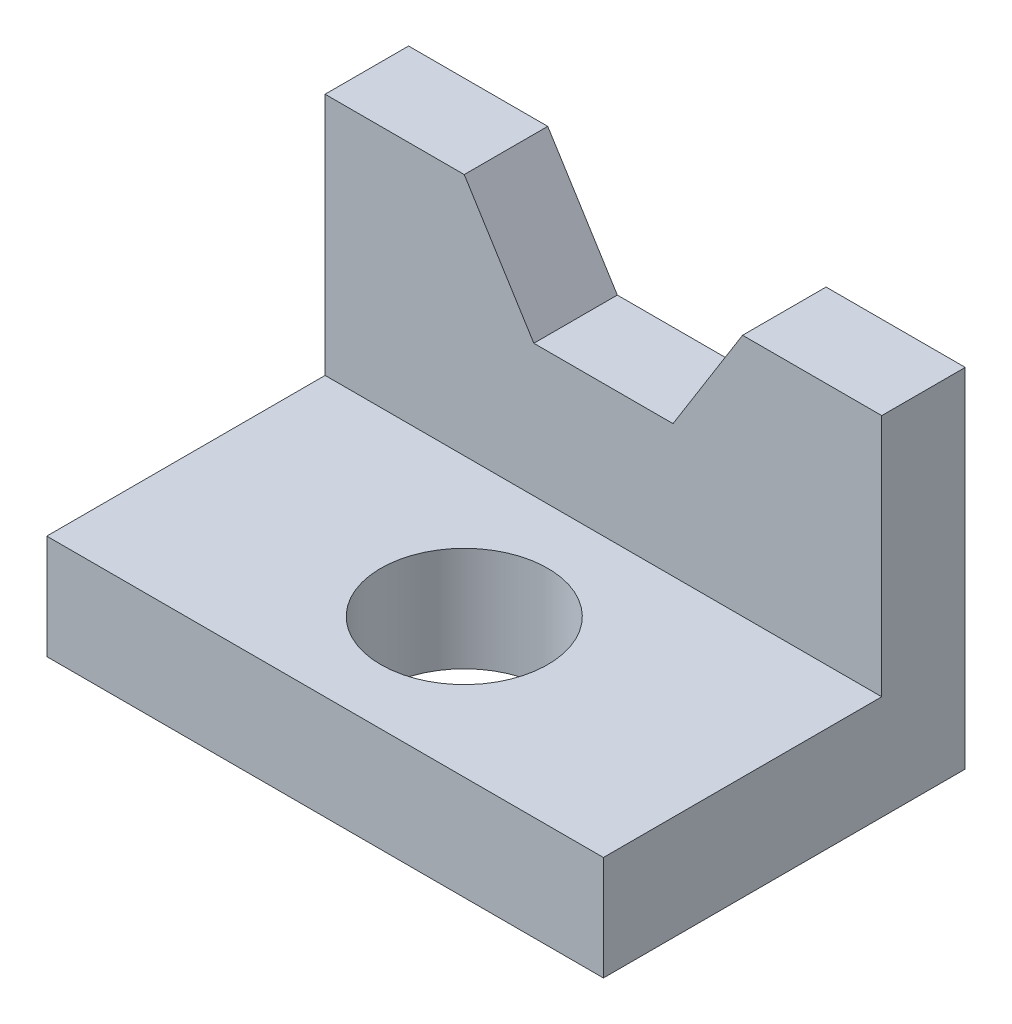
ISO-10303-21;
HEADER;
FILE_DESCRIPTION(('STEP AP214'),'2;1');
FILE_NAME('part.step','',(''),(''),'','','');
FILE_SCHEMA(('AUTOMOTIVE_DESIGN { 1 0 10303 214 1 1 1 1 }'));
ENDSEC;
DATA;
#1=APPLICATION_CONTEXT('core data for automotive mechanical design processes');
#2=APPLICATION_PROTOCOL_DEFINITION('international standard','automotive_design',2000,#1);
#3=PRODUCT_CONTEXT('',#1,'mechanical');
#4=PRODUCT('Part','Part','',(#3));
#5=PRODUCT_RELATED_PRODUCT_CATEGORY('part','',(#4));
#6=PRODUCT_DEFINITION_FORMATION('','',#4);
#7=PRODUCT_DEFINITION_CONTEXT('part definition',#1,'design');
#8=PRODUCT_DEFINITION('design','',#6,#7);
#9=PRODUCT_DEFINITION_SHAPE('','',#8);
#10=(LENGTH_UNIT() NAMED_UNIT(*) SI_UNIT(.MILLI.,.METRE.));
#11=(NAMED_UNIT(*) PLANE_ANGLE_UNIT() SI_UNIT($,.RADIAN.));
#12=(NAMED_UNIT(*) SI_UNIT($,.STERADIAN.) SOLID_ANGLE_UNIT());
#13=UNCERTAINTY_MEASURE_WITH_UNIT(LENGTH_MEASURE(1.E-05),#10,'distance_accuracy_value','');
#14=(GEOMETRIC_REPRESENTATION_CONTEXT(3) GLOBAL_UNCERTAINTY_ASSIGNED_CONTEXT((#13)) GLOBAL_UNIT_ASSIGNED_CONTEXT((#10,
#11,#12)) REPRESENTATION_CONTEXT('',''));
#15=CARTESIAN_POINT('',(0.,0.,0.));
#16=DIRECTION('',(0.,0.,1.));
#17=DIRECTION('',(1.,0.,0.));
#18=AXIS2_PLACEMENT_3D('',#15,#16,#17);
#19=CARTESIAN_POINT('',(0.,0.,12.));
#20=DIRECTION('',(0.,-1.,0.));
#21=DIRECTION('',(0.,0.,-1.));
#22=AXIS2_PLACEMENT_3D('',#19,#20,#21);
#23=PLANE('',#22);
#24=DIRECTION('',(-1.,0.,0.));
#25=VECTOR('',#24,1.);
#26=CARTESIAN_POINT('',(0.,0.,0.));
#27=LINE('',#26,#25);
#28=CARTESIAN_POINT('',(20.,0.,0.));
#29=VERTEX_POINT('',#28);
#30=CARTESIAN_POINT('',(0.,0.,0.));
#31=VERTEX_POINT('',#30);
#32=EDGE_CURVE('E143',#29,#31,#27,.T.);
#33=ORIENTED_EDGE('',*,*,#32,.T.);
#34=DIRECTION('',(0.,0.,-1.));
#35=VECTOR('',#34,1.);
#36=CARTESIAN_POINT('',(0.,0.,12.));
#37=LINE('',#36,#35);
#38=CARTESIAN_POINT('',(0.,0.,12.));
#39=VERTEX_POINT('',#38);
#40=EDGE_CURVE('E11',#39,#31,#37,.T.);
#41=ORIENTED_EDGE('',*,*,#40,.F.);
#42=DIRECTION('',(-1.,0.,0.));
#43=VECTOR('',#42,1.);
#44=CARTESIAN_POINT('',(0.,0.,12.));
#45=LINE('',#44,#43);
#46=CARTESIAN_POINT('',(20.,0.,12.));
#47=VERTEX_POINT('',#46);
#48=EDGE_CURVE('E160',#47,#39,#45,.T.);
#49=ORIENTED_EDGE('',*,*,#48,.F.);
#50=DIRECTION('',(0.,0.,-1.));
#51=VECTOR('',#50,1.);
#52=CARTESIAN_POINT('',(20.,0.,12.));
#53=LINE('',#52,#51);
#54=EDGE_CURVE('E140',#47,#29,#53,.T.);
#55=ORIENTED_EDGE('',*,*,#54,.T.);
#56=EDGE_LOOP('',(#33,#41,#49,#55));
#57=FACE_BOUND('',#56,.T.);
#58=ADVANCED_FACE('F41',(#57),#23,.F.);
#59=CARTESIAN_POINT('',(0.,0.,12.));
#60=DIRECTION('',(1.,0.,0.));
#61=DIRECTION('',(0.,0.,-1.));
#62=AXIS2_PLACEMENT_3D('',#59,#60,#61);
#63=PLANE('',#62);
#64=DIRECTION('',(0.,-1.,0.));
#65=VECTOR('',#64,1.);
#66=CARTESIAN_POINT('',(0.,0.,0.));
#67=LINE('',#66,#65);
#68=CARTESIAN_POINT('',(0.,-50.,0.));
#69=VERTEX_POINT('',#68);
#70=EDGE_CURVE('E145',#31,#69,#67,.T.);
#71=ORIENTED_EDGE('',*,*,#70,.T.);
#72=DIRECTION('',(0.,0.,-1.));
#73=VECTOR('',#72,1.);
#74=CARTESIAN_POINT('',(0.,-50.,12.));
#75=LINE('',#74,#73);
#76=CARTESIAN_POINT('',(0.,-50.,52.));
#77=VERTEX_POINT('',#76);
#78=EDGE_CURVE('E48',#77,#69,#75,.T.);
#79=ORIENTED_EDGE('',*,*,#78,.F.);
#80=DIRECTION('',(0.,-1.,0.));
#81=VECTOR('',#80,1.);
#82=CARTESIAN_POINT('',(0.,-50.,52.));
#83=LINE('',#82,#81);
#84=CARTESIAN_POINT('',(0.,-35.,52.));
#85=VERTEX_POINT('',#84);
#86=EDGE_CURVE('E199',#85,#77,#83,.T.);
#87=ORIENTED_EDGE('',*,*,#86,.F.);
#88=DIRECTION('',(0.,0.,-1.));
#89=VECTOR('',#88,1.);
#90=CARTESIAN_POINT('',(0.,-35.,52.));
#91=LINE('',#90,#89);
#92=CARTESIAN_POINT('',(0.,-35.,12.));
#93=VERTEX_POINT('',#92);
#94=EDGE_CURVE('E198',#85,#93,#91,.T.);
#95=ORIENTED_EDGE('',*,*,#94,.T.);
#96=DIRECTION('',(0.,-1.,0.));
#97=VECTOR('',#96,1.);
#98=CARTESIAN_POINT('',(0.,0.,12.));
#99=LINE('',#98,#97);
#100=EDGE_CURVE('E103',#39,#93,#99,.T.);
#101=ORIENTED_EDGE('',*,*,#100,.F.);
#102=ORIENTED_EDGE('',*,*,#40,.T.);
#103=EDGE_LOOP('',(#71,#79,#87,#95,#101,#102));
#104=FACE_BOUND('',#103,.T.);
#105=ADVANCED_FACE('F226',(#104),#63,.F.);
#106=CARTESIAN_POINT('',(0.,-50.,12.));
#107=DIRECTION('',(0.,1.,0.));
#108=DIRECTION('',(0.,0.,1.));
#109=AXIS2_PLACEMENT_3D('',#106,#107,#108);
#110=PLANE('',#109);
#111=CARTESIAN_POINT('',(40.,-50.,32.));
#112=DIRECTION('',(0.,1.,0.));
#113=DIRECTION('',(0.,0.,1.));
#114=AXIS2_PLACEMENT_3D('',#111,#112,#113);
#115=CIRCLE('',#114,12.);
#116=CARTESIAN_POINT('',(40.,-50.,44.));
#117=VERTEX_POINT('',#116);
#118=EDGE_CURVE('E203',#117,#117,#115,.T.);
#119=ORIENTED_EDGE('',*,*,#118,.T.);
#120=EDGE_LOOP('',(#119));
#121=FACE_BOUND('',#120,.T.);
#122=DIRECTION('',(1.,0.,0.));
#123=VECTOR('',#122,1.);
#124=CARTESIAN_POINT('',(0.,-50.,0.));
#125=LINE('',#124,#123);
#126=CARTESIAN_POINT('',(80.,-50.,0.));
#127=VERTEX_POINT('',#126);
#128=EDGE_CURVE('E150',#69,#127,#125,.T.);
#129=ORIENTED_EDGE('',*,*,#128,.T.);
#130=DIRECTION('',(0.,0.,-1.));
#131=VECTOR('',#130,1.);
#132=CARTESIAN_POINT('',(80.,-50.,12.));
#133=LINE('',#132,#131);
#134=CARTESIAN_POINT('',(80.,-50.,52.));
#135=VERTEX_POINT('',#134);
#136=EDGE_CURVE('E163',#135,#127,#133,.T.);
#137=ORIENTED_EDGE('',*,*,#136,.F.);
#138=DIRECTION('',(1.,0.,0.));
#139=VECTOR('',#138,1.);
#140=CARTESIAN_POINT('',(0.,-50.,52.));
#141=LINE('',#140,#139);
#142=EDGE_CURVE('E174',#77,#135,#141,.T.);
#143=ORIENTED_EDGE('',*,*,#142,.F.);
#144=ORIENTED_EDGE('',*,*,#78,.T.);
#145=EDGE_LOOP('',(#129,#137,#143,#144));
#146=FACE_BOUND('',#145,.T.);
#147=ADVANCED_FACE('F171',(#121,#146),#110,.F.);
#148=CARTESIAN_POINT('',(80.,-50.,12.));
#149=DIRECTION('',(-1.,0.,0.));
#150=DIRECTION('',(0.,0.,1.));
#151=AXIS2_PLACEMENT_3D('',#148,#149,#150);
#152=PLANE('',#151);
#153=DIRECTION('',(0.,1.,0.));
#154=VECTOR('',#153,1.);
#155=CARTESIAN_POINT('',(80.,-50.,0.));
#156=LINE('',#155,#154);
#157=CARTESIAN_POINT('',(80.,0.,0.));
#158=VERTEX_POINT('',#157);
#159=EDGE_CURVE('E149',#127,#158,#156,.T.);
#160=ORIENTED_EDGE('',*,*,#159,.T.);
#161=DIRECTION('',(0.,0.,-1.));
#162=VECTOR('',#161,1.);
#163=CARTESIAN_POINT('',(80.,0.,12.));
#164=LINE('',#163,#162);
#165=CARTESIAN_POINT('',(80.,0.,12.));
#166=VERTEX_POINT('',#165);
#167=EDGE_CURVE('E161',#166,#158,#164,.T.);
#168=ORIENTED_EDGE('',*,*,#167,.F.);
#169=DIRECTION('',(0.,1.,0.));
#170=VECTOR('',#169,1.);
#171=CARTESIAN_POINT('',(80.,-50.,12.));
#172=LINE('',#171,#170);
#173=CARTESIAN_POINT('',(80.,-35.,12.));
#174=VERTEX_POINT('',#173);
#175=EDGE_CURVE('E188',#174,#166,#172,.T.);
#176=ORIENTED_EDGE('',*,*,#175,.F.);
#177=DIRECTION('',(0.,0.,-1.));
#178=VECTOR('',#177,1.);
#179=CARTESIAN_POINT('',(80.,-35.,52.));
#180=LINE('',#179,#178);
#181=CARTESIAN_POINT('',(80.,-35.,52.));
#182=VERTEX_POINT('',#181);
#183=EDGE_CURVE('E144',#182,#174,#180,.T.);
#184=ORIENTED_EDGE('',*,*,#183,.F.);
#185=DIRECTION('',(0.,1.,0.));
#186=VECTOR('',#185,1.);
#187=CARTESIAN_POINT('',(80.,-50.,52.));
#188=LINE('',#187,#186);
#189=EDGE_CURVE('E204',#135,#182,#188,.T.);
#190=ORIENTED_EDGE('',*,*,#189,.F.);
#191=ORIENTED_EDGE('',*,*,#136,.T.);
#192=EDGE_LOOP('',(#160,#168,#176,#184,#190,#191));
#193=FACE_BOUND('',#192,.T.);
#194=ADVANCED_FACE('F183',(#193),#152,.F.);
#195=CARTESIAN_POINT('',(80.,0.,12.));
#196=DIRECTION('',(0.,-1.,0.));
#197=DIRECTION('',(0.,0.,-1.));
#198=AXIS2_PLACEMENT_3D('',#195,#196,#197);
#199=PLANE('',#198);
#200=DIRECTION('',(-1.,0.,0.));
#201=VECTOR('',#200,1.);
#202=CARTESIAN_POINT('',(80.,0.,0.));
#203=LINE('',#202,#201);
#204=CARTESIAN_POINT('',(60.,0.,0.));
#205=VERTEX_POINT('',#204);
#206=EDGE_CURVE('E151',#158,#205,#203,.T.);
#207=ORIENTED_EDGE('',*,*,#206,.T.);
#208=DIRECTION('',(0.,0.,-1.));
#209=VECTOR('',#208,1.);
#210=CARTESIAN_POINT('',(60.,0.,12.));
#211=LINE('',#210,#209);
#212=CARTESIAN_POINT('',(60.,0.,12.));
#213=VERTEX_POINT('',#212);
#214=EDGE_CURVE('E135',#213,#205,#211,.T.);
#215=ORIENTED_EDGE('',*,*,#214,.F.);
#216=DIRECTION('',(-1.,0.,0.));
#217=VECTOR('',#216,1.);
#218=CARTESIAN_POINT('',(80.,0.,12.));
#219=LINE('',#218,#217);
#220=EDGE_CURVE('E119',#166,#213,#219,.T.);
#221=ORIENTED_EDGE('',*,*,#220,.F.);
#222=ORIENTED_EDGE('',*,*,#167,.T.);
#223=EDGE_LOOP('',(#207,#215,#221,#222));
#224=FACE_BOUND('',#223,.T.);
#225=ADVANCED_FACE('F187',(#224),#199,.F.);
#226=CARTESIAN_POINT('',(50.,-16.,12.));
#227=DIRECTION('',(0.847998304005088,-0.52999894000318,0.));
#228=DIRECTION('',(0.52999894000318,0.847998304005088,0.));
#229=AXIS2_PLACEMENT_3D('',#226,#227,#228);
#230=PLANE('',#229);
#231=DIRECTION('',(-0.52999894000318,-0.847998304005088,0.));
#232=VECTOR('',#231,1.);
#233=CARTESIAN_POINT('',(50.,-16.,0.));
#234=LINE('',#233,#232);
#235=CARTESIAN_POINT('',(50.,-16.,0.));
#236=VERTEX_POINT('',#235);
#237=EDGE_CURVE('E129',#205,#236,#234,.T.);
#238=ORIENTED_EDGE('',*,*,#237,.T.);
#239=DIRECTION('',(0.,0.,-1.));
#240=VECTOR('',#239,1.);
#241=CARTESIAN_POINT('',(50.,-16.,12.));
#242=LINE('',#241,#240);
#243=CARTESIAN_POINT('',(50.,-16.,12.));
#244=VERTEX_POINT('',#243);
#245=EDGE_CURVE('E127',#244,#236,#242,.T.);
#246=ORIENTED_EDGE('',*,*,#245,.F.);
#247=DIRECTION('',(-0.52999894000318,-0.847998304005088,0.));
#248=VECTOR('',#247,1.);
#249=CARTESIAN_POINT('',(50.,-16.,12.));
#250=LINE('',#249,#248);
#251=EDGE_CURVE('E114',#213,#244,#250,.T.);
#252=ORIENTED_EDGE('',*,*,#251,.F.);
#253=ORIENTED_EDGE('',*,*,#214,.T.);
#254=EDGE_LOOP('',(#238,#246,#252,#253));
#255=FACE_BOUND('',#254,.T.);
#256=ADVANCED_FACE('F130',(#255),#230,.F.);
#257=CARTESIAN_POINT('',(50.,-16.,12.));
#258=DIRECTION('',(0.,-1.,0.));
#259=DIRECTION('',(0.,0.,-1.));
#260=AXIS2_PLACEMENT_3D('',#257,#258,#259);
#261=PLANE('',#260);
#262=DIRECTION('',(-1.,0.,0.));
#263=VECTOR('',#262,1.);
#264=CARTESIAN_POINT('',(50.,-16.,0.));
#265=LINE('',#264,#263);
#266=CARTESIAN_POINT('',(30.,-16.,0.));
#267=VERTEX_POINT('',#266);
#268=EDGE_CURVE('E152',#236,#267,#265,.T.);
#269=ORIENTED_EDGE('',*,*,#268,.T.);
#270=DIRECTION('',(0.,0.,-1.));
#271=VECTOR('',#270,1.);
#272=CARTESIAN_POINT('',(30.,-16.,12.));
#273=LINE('',#272,#271);
#274=CARTESIAN_POINT('',(30.,-16.,12.));
#275=VERTEX_POINT('',#274);
#276=EDGE_CURVE('E132',#275,#267,#273,.T.);
#277=ORIENTED_EDGE('',*,*,#276,.F.);
#278=DIRECTION('',(-1.,0.,0.));
#279=VECTOR('',#278,1.);
#280=CARTESIAN_POINT('',(50.,-16.,12.));
#281=LINE('',#280,#279);
#282=EDGE_CURVE('E120',#244,#275,#281,.T.);
#283=ORIENTED_EDGE('',*,*,#282,.F.);
#284=ORIENTED_EDGE('',*,*,#245,.T.);
#285=EDGE_LOOP('',(#269,#277,#283,#284));
#286=FACE_BOUND('',#285,.T.);
#287=ADVANCED_FACE('F134',(#286),#261,.F.);
#288=CARTESIAN_POINT('',(20.,0.,12.));
#289=DIRECTION('',(-0.847998304005088,-0.52999894000318,0.));
#290=DIRECTION('',(0.52999894000318,-0.847998304005088,0.));
#291=AXIS2_PLACEMENT_3D('',#288,#289,#290);
#292=PLANE('',#291);
#293=DIRECTION('',(-0.52999894000318,0.847998304005088,0.));
#294=VECTOR('',#293,1.);
#295=CARTESIAN_POINT('',(20.,0.,0.));
#296=LINE('',#295,#294);
#297=EDGE_CURVE('E96',#267,#29,#296,.T.);
#298=ORIENTED_EDGE('',*,*,#297,.T.);
#299=ORIENTED_EDGE('',*,*,#54,.F.);
#300=DIRECTION('',(-0.52999894000318,0.847998304005088,0.));
#301=VECTOR('',#300,1.);
#302=CARTESIAN_POINT('',(20.,0.,12.));
#303=LINE('',#302,#301);
#304=EDGE_CURVE('E62',#275,#47,#303,.T.);
#305=ORIENTED_EDGE('',*,*,#304,.F.);
#306=ORIENTED_EDGE('',*,*,#276,.T.);
#307=EDGE_LOOP('',(#298,#299,#305,#306));
#308=FACE_BOUND('',#307,.T.);
#309=ADVANCED_FACE('F247',(#308),#292,.F.);
#310=CARTESIAN_POINT('',(0.,0.,12.));
#311=DIRECTION('',(0.,0.,1.));
#312=DIRECTION('',(1.,0.,0.));
#313=AXIS2_PLACEMENT_3D('',#310,#311,#312);
#314=PLANE('',#313);
#315=DIRECTION('',(-1.,0.,0.));
#316=VECTOR('',#315,1.);
#317=CARTESIAN_POINT('',(0.,-35.,12.));
#318=LINE('',#317,#316);
#319=EDGE_CURVE('E54',#174,#93,#318,.T.);
#320=ORIENTED_EDGE('',*,*,#319,.F.);
#321=ORIENTED_EDGE('',*,*,#175,.T.);
#322=ORIENTED_EDGE('',*,*,#220,.T.);
#323=ORIENTED_EDGE('',*,*,#251,.T.);
#324=ORIENTED_EDGE('',*,*,#282,.T.);
#325=ORIENTED_EDGE('',*,*,#304,.T.);
#326=ORIENTED_EDGE('',*,*,#48,.T.);
#327=ORIENTED_EDGE('',*,*,#100,.T.);
#328=EDGE_LOOP('',(#320,#321,#322,#323,#324,#325,#326,#327));
#329=FACE_BOUND('',#328,.T.);
#330=ADVANCED_FACE('F113',(#329),#314,.T.);
#331=CARTESIAN_POINT('',(0.,0.,0.));
#332=DIRECTION('',(0.,0.,1.));
#333=DIRECTION('',(1.,0.,0.));
#334=AXIS2_PLACEMENT_3D('',#331,#332,#333);
#335=PLANE('',#334);
#336=ORIENTED_EDGE('',*,*,#32,.F.);
#337=ORIENTED_EDGE('',*,*,#297,.F.);
#338=ORIENTED_EDGE('',*,*,#268,.F.);
#339=ORIENTED_EDGE('',*,*,#237,.F.);
#340=ORIENTED_EDGE('',*,*,#206,.F.);
#341=ORIENTED_EDGE('',*,*,#159,.F.);
#342=ORIENTED_EDGE('',*,*,#128,.F.);
#343=ORIENTED_EDGE('',*,*,#70,.F.);
#344=EDGE_LOOP('',(#336,#337,#338,#339,#340,#341,#342,#343));
#345=FACE_BOUND('',#344,.T.);
#346=ADVANCED_FACE('F182',(#345),#335,.F.);
#347=CARTESIAN_POINT('',(0.,-35.,52.));
#348=DIRECTION('',(0.,-1.,0.));
#349=DIRECTION('',(0.,0.,-1.));
#350=AXIS2_PLACEMENT_3D('',#347,#348,#349);
#351=PLANE('',#350);
#352=CARTESIAN_POINT('',(40.,-35.,32.));
#353=DIRECTION('',(0.,1.,0.));
#354=DIRECTION('',(0.,0.,1.));
#355=AXIS2_PLACEMENT_3D('',#352,#353,#354);
#356=CIRCLE('',#355,12.);
#357=CARTESIAN_POINT('',(40.,-35.,44.));
#358=VERTEX_POINT('',#357);
#359=EDGE_CURVE('E211',#358,#358,#356,.T.);
#360=ORIENTED_EDGE('',*,*,#359,.F.);
#361=EDGE_LOOP('',(#360));
#362=FACE_BOUND('',#361,.T.);
#363=ORIENTED_EDGE('',*,*,#319,.T.);
#364=ORIENTED_EDGE('',*,*,#94,.F.);
#365=DIRECTION('',(-1.,0.,0.));
#366=VECTOR('',#365,1.);
#367=CARTESIAN_POINT('',(0.,-35.,52.));
#368=LINE('',#367,#366);
#369=EDGE_CURVE('E196',#182,#85,#368,.T.);
#370=ORIENTED_EDGE('',*,*,#369,.F.);
#371=ORIENTED_EDGE('',*,*,#183,.T.);
#372=EDGE_LOOP('',(#363,#364,#370,#371));
#373=FACE_BOUND('',#372,.T.);
#374=ADVANCED_FACE('F217',(#362,#373),#351,.F.);
#375=CARTESIAN_POINT('',(0.,0.,52.));
#376=DIRECTION('',(0.,0.,-1.));
#377=DIRECTION('',(-1.,0.,0.));
#378=AXIS2_PLACEMENT_3D('',#375,#376,#377);
#379=PLANE('',#378);
#380=ORIENTED_EDGE('',*,*,#86,.T.);
#381=ORIENTED_EDGE('',*,*,#142,.T.);
#382=ORIENTED_EDGE('',*,*,#189,.T.);
#383=ORIENTED_EDGE('',*,*,#369,.T.);
#384=EDGE_LOOP('',(#380,#381,#382,#383));
#385=FACE_BOUND('',#384,.T.);
#386=ADVANCED_FACE('F222',(#385),#379,.F.);
#387=CARTESIAN_POINT('',(40.,-55.,32.));
#388=DIRECTION('',(0.,1.,0.));
#389=DIRECTION('',(0.,0.,1.));
#390=AXIS2_PLACEMENT_3D('',#387,#388,#389);
#391=CYLINDRICAL_SURFACE('',#390,12.);
#392=ORIENTED_EDGE('',*,*,#359,.T.);
#393=EDGE_LOOP('',(#392));
#394=FACE_BOUND('',#393,.T.);
#395=ORIENTED_EDGE('',*,*,#118,.F.);
#396=EDGE_LOOP('',(#395));
#397=FACE_BOUND('',#396,.T.);
#398=ADVANCED_FACE('F214',(#394,#397),#391,.F.);
#399=CLOSED_SHELL('',(#58,#105,#147,#194,#225,#256,#287,#309,#330,#346,#374,#386,#398));
#400=MANIFOLD_SOLID_BREP('B2',#399);
#401=ADVANCED_BREP_SHAPE_REPRESENTATION('',(#18,#400),#14);
#402=SHAPE_DEFINITION_REPRESENTATION(#9,#401);
ENDSEC;
END-ISO-10303-21;
